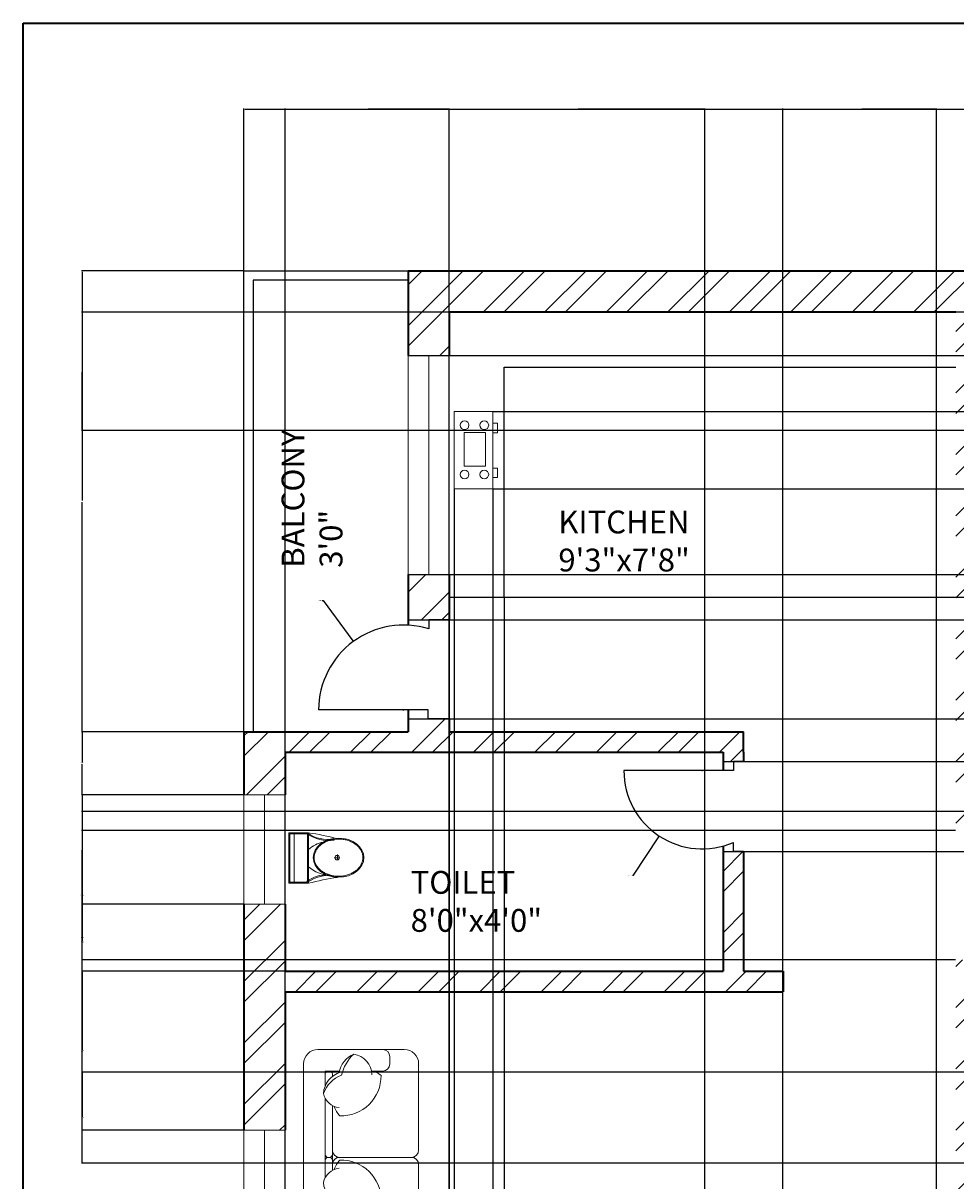
# Model space of a CAD drawing. Units: inches. Extents: x 2529 to 3014, y 1203 to 2262.
# Tile 10 of 13: x 2529 to 2733, y 2008 to 2262. Entities that reach past the tile are written whole.
import ezdxf

# ---------------------------------------------------------------- set-up
doc = ezdxf.new("R2010")
doc.units = ezdxf.units.IN
for name, color, linetype, lineweight in [('A-ANNO-DIMS', 2, 'Continuous', 18), ('A-ANNO-TTLB', 7, 'Continuous', 35), ('A-AREA-IDEN', 7, 'Continuous', 18), ('A-DOOR', 21, 'Continuous', 25), ('A-EQPM', 8, 'Continuous', 18), ('A-FLOR-CASE', 7, 'Continuous', 25), ('A-FLOR-FIXT', 8, 'Continuous', 18), ('A-FLOR-RAIL', 61, 'Continuous', 25), ('A-FURN', 8, 'Continuous', 18), ('A-GLAZ', 191, 'Continuous', 18), ('A-WALL', 7, 'Continuous', 35), ('A-WALL-PATT', 143, 'Continuous', 13)]:
    doc.layers.add(name, color=color, linetype=linetype, lineweight=lineweight)
doc.styles.get("Standard").update_dxf_attribs({"font": 'arial.ttf'})
doc.dimstyles.get("Standard").update_dxf_attribs({"dimtxt": 0.18, "dimasz": 0.18, "dimexe": 0.18, "dimexo": 0.0625, "dimgap": 0.09, "dimtad": 0, "dimtih": 1, "dimtoh": 1, "dimdec": 4, "dimzin": 0, "dimdsep": 46, "dimtxsty": 'Standard', "dimcen": 0.09, "dimadec": 0, "dimazin": 0, "dimtfac": 1, "dimtdec": 4, "dimtofl": 0, "dimtmove": 0, "dimatfit": 3, "dimfxl": 1, "dimtolj": 1, "dimtzin": 0, "dimarcsym": 0})

# ---------------------------------------------------------------- blocks, each defined once
blk = doc.blocks.new('A$C31115884')
for p, q in [((283, 498), (223, 498)), ((258, 466), (258, 523)), ((0, 200), (0, 0)), ((520, 200), (0, 200)), ((10, 190), (10, 10)), ((510, 190), (10, 190)), ((510, 10), (510, 190)), ((520, 0), (520, 200)), ((510, 54), (0, 54)), ((10, 10), (510, 10)), ((0, 0), (520, 0))]:
    blk.add_line(p, q)
blk.add_circle((256, 496), 23.6)
for centre, radius, start, end in [((2778, -205), 2807, 165.4549, 171.7133), ((3237, 905), 2807, 188.2867, 194.5451), ((-295, 403), 365, 324.2091, 9.3499), ((-295, 403), 375, 324.2091, 9.3499), ((139, 406), 293, 315.8436, 2.6563), ((806, 403), 375, 179.2036, 215.7909), ((806, 403), 365, 170.6501, 215.7909), ((384, 406), 293, 190.2774, 224.1564)]:
    blk.add_arc(centre, radius, start, end)
blk.add_ellipse((256, 510), major_axis=(0, -261), ratio=0.772727)
blk.add_open_spline([(256, 259), (263, 259), (270, 260), (288, 262), (299, 265), (320, 273), (330, 278), (350, 291), (360, 299), (378, 316), (386, 326), (402, 347), (409, 358), (421, 383), (427, 395), (436, 422), (440, 436), (445, 465), (447, 480), (448, 509), (448, 524), (445, 553), (443, 568), (436, 596), (432, 610), (422, 636), (416, 649), (402, 672), (395, 683), (379, 703), (370, 712), (351, 728), (341, 735), (321, 746), (310, 751), (289, 757), (278, 759), (256, 761), (245, 761), (223, 757), (212, 754), (191, 746), (181, 741), (161, 728), (151, 720), (133, 703), (125, 693), (110, 672), (103, 660), (90, 636), (85, 623), (76, 596), (72, 582), (67, 553), (66, 538), (64, 509), (65, 494), (68, 465), (70, 450), (77, 422), (81, 408), (91, 382), (97, 370), (111, 346), (118, 335), (135, 316), (144, 307), (162, 291), (172, 284), (193, 273), (203, 269), (225, 262), (236, 260), (250, 259), (253, 259), (256, 259)], degree=3, knots=[0, 0, 0, 0, 0.110105, 0.110105, 0.285049, 0.285049, 0.459994, 0.459994, 0.634938, 0.634938, 0.809882, 0.809882, 0.984827, 0.984827, 1.159771, 1.159771, 1.334715, 1.334715, 1.50966, 1.50966, 1.684604, 1.684604, 1.859549, 1.859549, 2.034493, 2.034493, 2.209437, 2.209437, 2.384382, 2.384382, 2.559326, 2.559326, 2.73427, 2.73427, 2.909215, 2.909215, 3.084159, 3.084159, 3.259103, 3.259103, 3.434048, 3.434048, 3.608992, 3.608992, 3.783936, 3.783936, 3.958881, 3.958881, 4.133825, 4.133825, 4.30877, 4.30877, 4.483714, 4.483714, 4.658658, 4.658658, 4.833603, 4.833603, 5.008547, 5.008547, 5.183491, 5.183491, 5.358436, 5.358436, 5.53338, 5.53338, 5.708324, 5.708324, 5.883269, 5.883269, 6.058213, 6.058213, 6.233158, 6.233158, 6.283185, 6.283185, 6.283185, 6.283185])
blk = doc.blocks.new('WIN-60x9')
for p, q in [((0, 60), (9, 60)), ((0, 60), (0, 0)), ((9, 60), (4.5, 60)), ((4.5, 60), (4.5, 0)), ((9, 60), (9, 0)), ((4.5, 0), (0, 0)), ((0, 0), (9, 0))]:
    blk.add_line(p, q)
blk = doc.blocks.new('*D16')
at = {"layer": 'A-ANNO-DIMS', "color": 0, "lineweight": -2, "transparency": 16777216}
for p, q in [((2577.06, 2207.57), (2577.06, 2243.11)), ((2577.24, 2242.93), (2774.27, 2242.93)), ((2971.88, 2242.93), (2774.84, 2242.93)), ((2972.06, 2207.57), (2972.06, 2243.11))]:
    blk.add_line(p, q, dxfattribs=at)
at = {"layer": 'A-ANNO-DIMS', "color": 0, "transparency": 16777216}
for points in [[(2577.24, 2242.96), (2577.24, 2242.9), (2577.06, 2242.93)], [(2971.88, 2242.96), (2971.88, 2242.9), (2972.06, 2242.93)]]:
    blk.add_solid(points, dxfattribs=at)
at = {"layer": 'Defpoints', "color": 0, "transparency": 16777216}
for p in [(2972.06, 2242.93), (2577.06, 2207.5), (2972.06, 2207.5)]:
    blk.add_point(p, dxfattribs=at)
at = {"layer": 'A-ANNO-DIMS', "color": 0, "transparency": 16777216, "insert": (2774.56, 2242.93), "char_height": 0.18, "attachment_point": 5}
blk.add_mtext('\\A1;395', dxfattribs=at)
blk = doc.blocks.new('*D27')
at = {"layer": 'A-ANNO-DIMS', "color": 0, "lineweight": -2, "transparency": 16777216}
for p, q in [((2585.99, 2054), (2541.45, 2054)), ((2541.63, 2053.82), (2541.63, 2036.75)), ((2541.63, 2019.3), (2541.63, 2036.38)), ((2576.99, 2019.12), (2541.45, 2019.12))]:
    blk.add_line(p, q, dxfattribs=at)
at = {"layer": 'A-ANNO-DIMS', "color": 0, "transparency": 16777216}
for points in [[(2541.6, 2053.82), (2541.66, 2053.82), (2541.63, 2054)], [(2541.6, 2019.3), (2541.66, 2019.3), (2541.63, 2019.12)]]:
    blk.add_solid(points, dxfattribs=at)
at = {"layer": 'Defpoints', "color": 0, "transparency": 16777216}
for p in [(2541.63, 2054), (2586.06, 2054), (2577.06, 2019.12)]:
    blk.add_point(p, dxfattribs=at)
at = {"layer": 'A-ANNO-DIMS', "color": 0, "transparency": 16777216, "insert": (2541.63, 2036.56), "char_height": 0.18, "attachment_point": 5}
blk.add_mtext('\\A1;34.88', dxfattribs=at)
blk = doc.blocks.new('*D28')
at = {"layer": 'A-ANNO-DIMS', "color": 0, "lineweight": -2, "transparency": 16777216}
for p, q in [((2576.99, 2068.69), (2541.45, 2068.69)), ((2541.63, 2068.51), (2541.63, 2061.53)), ((2541.63, 2054.18), (2541.63, 2061.17)), ((2585.99, 2054), (2541.45, 2054))]:
    blk.add_line(p, q, dxfattribs=at)
at = {"layer": 'A-ANNO-DIMS', "color": 0, "transparency": 16777216}
for points in [[(2541.6, 2068.51), (2541.66, 2068.51), (2541.63, 2068.69)], [(2541.6, 2054.18), (2541.66, 2054.18), (2541.63, 2054)]]:
    blk.add_solid(points, dxfattribs=at)
at = {"layer": 'Defpoints', "color": 0, "transparency": 16777216}
for p in [(2541.63, 2068.69), (2577.06, 2068.69), (2586.06, 2054)]:
    blk.add_point(p, dxfattribs=at)
at = {"layer": 'A-ANNO-DIMS', "color": 0, "transparency": 16777216, "insert": (2541.63, 2061.35), "char_height": 0.18, "attachment_point": 5}
blk.add_mtext('\\A1;14.69', dxfattribs=at)
blk = doc.blocks.new('*D29')
at = {"layer": 'A-ANNO-DIMS', "color": 0, "lineweight": -2, "transparency": 16777216}
for p, q in [((2576.99, 2092.69), (2541.45, 2092.69)), ((2541.63, 2092.51), (2541.63, 2080.87)), ((2541.63, 2068.87), (2541.63, 2080.51)), ((2576.99, 2068.69), (2541.45, 2068.69))]:
    blk.add_line(p, q, dxfattribs=at)
at = {"layer": 'A-ANNO-DIMS', "color": 0, "transparency": 16777216}
for points in [[(2541.6, 2092.51), (2541.66, 2092.51), (2541.63, 2092.69)], [(2541.6, 2068.87), (2541.66, 2068.87), (2541.63, 2068.69)]]:
    blk.add_solid(points, dxfattribs=at)
at = {"layer": 'Defpoints', "color": 0, "transparency": 16777216}
for p in [(2541.63, 2092.69), (2577.06, 2092.69), (2577.06, 2068.69)]:
    blk.add_point(p, dxfattribs=at)
at = {"layer": 'A-ANNO-DIMS', "color": 0, "transparency": 16777216, "insert": (2541.63, 2080.69), "char_height": 0.18, "attachment_point": 5}
blk.add_mtext('\\A1;24', dxfattribs=at)
blk = doc.blocks.new('*D30')
at = {"layer": 'A-ANNO-DIMS', "color": 0, "lineweight": -2, "transparency": 16777216}
for p, q in [((2576.99, 2106.5), (2541.45, 2106.5)), ((2541.63, 2106.32), (2541.63, 2099.78)), ((2541.63, 2092.87), (2541.63, 2099.42)), ((2576.99, 2092.69), (2541.45, 2092.69))]:
    blk.add_line(p, q, dxfattribs=at)
at = {"layer": 'A-ANNO-DIMS', "color": 0, "transparency": 16777216}
for points in [[(2541.6, 2106.32), (2541.66, 2106.32), (2541.63, 2106.5)], [(2541.6, 2092.87), (2541.66, 2092.87), (2541.63, 2092.69)]]:
    blk.add_solid(points, dxfattribs=at)
at = {"layer": 'Defpoints', "color": 0, "transparency": 16777216}
for p in [(2541.63, 2106.5), (2577.06, 2106.5), (2577.06, 2092.69)]:
    blk.add_point(p, dxfattribs=at)
at = {"layer": 'A-ANNO-DIMS', "color": 0, "transparency": 16777216, "insert": (2541.63, 2099.6), "char_height": 0.18, "attachment_point": 5}
blk.add_mtext('\\A1;13.811', dxfattribs=at)
blk = doc.blocks.new('*D31')
at = {"layer": 'A-ANNO-DIMS', "color": 0, "lineweight": -2, "transparency": 16777216}
for p, q in [((2576.99, 2207.5), (2541.45, 2207.5)), ((2541.63, 2207.32), (2541.63, 2157.19)), ((2541.63, 2106.68), (2541.63, 2156.82)), ((2576.99, 2106.5), (2541.45, 2106.5))]:
    blk.add_line(p, q, dxfattribs=at)
at = {"layer": 'A-ANNO-DIMS', "color": 0, "transparency": 16777216}
for points in [[(2541.6, 2207.32), (2541.66, 2207.32), (2541.63, 2207.5)], [(2541.6, 2106.68), (2541.66, 2106.68), (2541.63, 2106.5)]]:
    blk.add_solid(points, dxfattribs=at)
at = {"layer": 'Defpoints', "color": 0, "transparency": 16777216}
for p in [(2541.63, 2207.5), (2577.06, 2207.5), (2577.06, 2106.5)]:
    blk.add_point(p, dxfattribs=at)
at = {"layer": 'A-ANNO-DIMS', "color": 0, "transparency": 16777216, "insert": (2541.63, 2157), "char_height": 0.18, "attachment_point": 5}
blk.add_mtext('\\A1;101', dxfattribs=at)
blk = doc.blocks.new('*D32')
at = {"layer": 'A-ANNO-DIMS', "color": 0, "lineweight": -2, "transparency": 16777216}
for p, q in [((2586.06, 1826.63), (2586.06, 2243.11)), ((2586.24, 2242.93), (2603.84, 2242.93)), ((2621.88, 2242.93), (2604.27, 2242.93)), ((2622.06, 1826.63), (2622.06, 2243.11))]:
    blk.add_line(p, q, dxfattribs=at)
at = {"layer": 'A-ANNO-DIMS', "color": 0, "transparency": 16777216}
for points in [[(2586.24, 2242.96), (2586.24, 2242.9), (2586.06, 2242.93)], [(2621.88, 2242.96), (2621.88, 2242.9), (2622.06, 2242.93)]]:
    blk.add_solid(points, dxfattribs=at)
at = {"layer": 'Defpoints', "color": 0, "transparency": 16777216}
for p in [(2622.06, 2242.93), (2586.06, 1826.57), (2622.06, 1826.57)]:
    blk.add_point(p, dxfattribs=at)
at = {"layer": 'A-ANNO-DIMS', "color": 0, "transparency": 16777216, "insert": (2604.06, 2242.93), "char_height": 0.18, "attachment_point": 5}
blk.add_mtext('\\A1;36', dxfattribs=at)
blk = doc.blocks.new('*D46')
at = {"layer": 'A-ANNO-DIMS', "color": 0, "lineweight": -2, "transparency": 16777216}
for p, q in [((2613.12, 2188.94), (3007.66, 2188.94)), ((3007.48, 2188.76), (3007.48, 2165.12)), ((3007.48, 2141.12), (3007.48, 2164.75)), ((2613.12, 2140.94), (3007.66, 2140.94))]:
    blk.add_line(p, q, dxfattribs=at)
at = {"layer": 'A-ANNO-DIMS', "color": 0, "transparency": 16777216}
for points in [[(3007.45, 2188.76), (3007.51, 2188.76), (3007.48, 2188.94)], [(3007.45, 2141.12), (3007.51, 2141.12), (3007.48, 2140.94)]]:
    blk.add_solid(points, dxfattribs=at)
at = {"layer": 'Defpoints', "color": 0, "transparency": 16777216}
for p in [(2613.06, 2188.94), (3007.48, 2188.94), (2613.06, 2140.94)]:
    blk.add_point(p, dxfattribs=at)
at = {"layer": 'A-ANNO-DIMS', "color": 0, "transparency": 16777216, "insert": (3007.48, 2164.94), "char_height": 0.18, "attachment_point": 5}
blk.add_mtext('\\A1;48', dxfattribs=at)
blk = doc.blocks.new('*D47')
at = {"layer": 'A-ANNO-DIMS', "color": 0, "lineweight": -2, "transparency": 16777216}
for p, q in [((2622.12, 2131.02), (3007.66, 2131.02)), ((3007.48, 2130.84), (3007.48, 2120.34)), ((3007.48, 2109.48), (3007.48, 2119.98)), ((2622.12, 2109.3), (3007.66, 2109.3))]:
    blk.add_line(p, q, dxfattribs=at)
at = {"layer": 'A-ANNO-DIMS', "color": 0, "transparency": 16777216}
for points in [[(3007.45, 2130.84), (3007.51, 2130.84), (3007.48, 2131.02)], [(3007.45, 2109.48), (3007.51, 2109.48), (3007.48, 2109.3)]]:
    blk.add_solid(points, dxfattribs=at)
at = {"layer": 'Defpoints', "color": 0, "transparency": 16777216}
for p in [(2622.06, 2131.02), (3007.48, 2131.02), (2622.06, 2109.3)]:
    blk.add_point(p, dxfattribs=at)
at = {"layer": 'A-ANNO-DIMS', "color": 0, "transparency": 16777216, "insert": (3007.48, 2120.16), "char_height": 0.18, "attachment_point": 5}
blk.add_mtext('\\A1;21.72', dxfattribs=at)
blk = doc.blocks.new('*D48')
at = {"layer": 'A-ANNO-DIMS', "color": 0, "lineweight": -2, "transparency": 16777216}
for p, q in [((2686.62, 2099.98), (3007.66, 2099.98)), ((3007.48, 2099.8), (3007.48, 2090.29)), ((3007.48, 2080.41), (3007.48, 2089.93)), ((2686.62, 2080.23), (3007.66, 2080.23))]:
    blk.add_line(p, q, dxfattribs=at)
at = {"layer": 'A-ANNO-DIMS', "color": 0, "transparency": 16777216}
for points in [[(3007.45, 2099.8), (3007.51, 2099.8), (3007.48, 2099.98)], [(3007.45, 2080.41), (3007.51, 2080.41), (3007.48, 2080.23)]]:
    blk.add_solid(points, dxfattribs=at)
at = {"layer": 'Defpoints', "color": 0, "transparency": 16777216}
for p in [(2686.56, 2099.98), (3007.48, 2099.98), (2686.56, 2080.23)]:
    blk.add_point(p, dxfattribs=at)
at = {"layer": 'A-ANNO-DIMS', "color": 0, "transparency": 16777216, "insert": (3007.48, 2090.11), "char_height": 0.18, "attachment_point": 5}
blk.add_mtext('\\A1;19.75', dxfattribs=at)
blk = doc.blocks.new('*D49')
at = {"layer": 'A-ANNO-DIMS', "color": 0, "lineweight": -2, "transparency": 16777216}
for p, q in [((2732.99, 2084.81), (2541.45, 2084.81)), ((2541.63, 2084.63), (2541.63, 2070.83)), ((2541.63, 2056.67), (2541.63, 2070.47)), ((2732.99, 2056.49), (2541.45, 2056.49))]:
    blk.add_line(p, q, dxfattribs=at)
at = {"layer": 'A-ANNO-DIMS', "color": 0, "transparency": 16777216}
for points in [[(2541.6, 2084.63), (2541.66, 2084.63), (2541.63, 2084.81)], [(2541.6, 2056.67), (2541.66, 2056.67), (2541.63, 2056.49)]]:
    blk.add_solid(points, dxfattribs=at)
at = {"layer": 'Defpoints', "color": 0, "transparency": 16777216}
for p in [(2541.63, 2084.81), (2733.06, 2084.81), (2733.06, 2056.49)]:
    blk.add_point(p, dxfattribs=at)
at = {"layer": 'A-ANNO-DIMS', "color": 0, "transparency": 16777216, "insert": (2541.63, 2070.65), "char_height": 0.18, "attachment_point": 5}
blk.add_mtext('\\A1;28.316', dxfattribs=at)
blk = doc.blocks.new('*D52')
at = {"layer": 'A-ANNO-DIMS', "color": 0, "lineweight": -2, "transparency": 16777216}
for p, q in [((2695.12, 1917.57), (2695.12, 2243.11)), ((2695.3, 2242.93), (2711.5, 2242.93)), ((2728.62, 2242.93), (2712.42, 2242.93)), ((2728.8, 1917.57), (2728.8, 2243.11))]:
    blk.add_line(p, q, dxfattribs=at)
at = {"layer": 'A-ANNO-DIMS', "color": 0, "transparency": 16777216}
for points in [[(2695.3, 2242.96), (2695.3, 2242.9), (2695.12, 2242.93)], [(2728.62, 2242.96), (2728.62, 2242.9), (2728.8, 2242.93)]]:
    blk.add_solid(points, dxfattribs=at)
at = {"layer": 'Defpoints', "color": 0, "transparency": 16777216}
for p in [(2728.8, 2242.93), (2695.12, 1917.5), (2728.8, 1917.5)]:
    blk.add_point(p, dxfattribs=at)
at = {"layer": 'A-ANNO-DIMS', "color": 0, "transparency": 16777216, "insert": (2711.96, 2242.93), "char_height": 0.18, "attachment_point": 5}
blk.add_mtext('\\A1;33.673', dxfattribs=at)
blk = doc.blocks.new('*D54')
at = {"layer": 'A-ANNO-DIMS', "color": 0, "lineweight": -2, "transparency": 16777216}
for p, q in [((2866.49, 2198.5), (2541.45, 2198.5)), ((2541.63, 2198.32), (2541.63, 2185.69)), ((2541.63, 2172.68), (2541.63, 2185.32)), ((2866.49, 2172.5), (2541.45, 2172.5))]:
    blk.add_line(p, q, dxfattribs=at)
at = {"layer": 'A-ANNO-DIMS', "color": 0, "transparency": 16777216}
for points in [[(2541.6, 2198.32), (2541.66, 2198.32), (2541.63, 2198.5)], [(2541.6, 2172.68), (2541.66, 2172.68), (2541.63, 2172.5)]]:
    blk.add_solid(points, dxfattribs=at)
at = {"layer": 'Defpoints', "color": 0, "transparency": 16777216}
for p in [(2541.63, 2198.5), (2866.56, 2198.5), (2866.56, 2172.5)]:
    blk.add_point(p, dxfattribs=at)
at = {"layer": 'A-ANNO-DIMS', "color": 0, "transparency": 16777216, "insert": (2541.63, 2185.5), "char_height": 0.18, "attachment_point": 5}
blk.add_mtext('\\A1;26', dxfattribs=at)
blk = doc.blocks.new('*D58')
at = {"layer": 'A-ANNO-DIMS', "color": 0, "lineweight": -2, "transparency": 16777216}
for p, q in [((2918.49, 2089), (2541.45, 2089)), ((2541.63, 2088.82), (2541.63, 2060.62)), ((2541.63, 2032.05), (2541.63, 2060.26)), ((2918.49, 2031.87), (2541.45, 2031.87))]:
    blk.add_line(p, q, dxfattribs=at)
at = {"layer": 'A-ANNO-DIMS', "color": 0, "transparency": 16777216}
for points in [[(2541.6, 2088.82), (2541.66, 2088.82), (2541.63, 2089)], [(2541.6, 2032.05), (2541.66, 2032.05), (2541.63, 2031.87)]]:
    blk.add_solid(points, dxfattribs=at)
at = {"layer": 'Defpoints', "color": 0, "transparency": 16777216}
for p in [(2918.56, 2089), (2541.63, 2031.87), (2918.56, 2031.87)]:
    blk.add_point(p, dxfattribs=at)
at = {"layer": 'A-ANNO-DIMS', "color": 0, "transparency": 16777216, "insert": (2541.63, 2060.44), "char_height": 0.18, "attachment_point": 5}
blk.add_mtext('\\A1;57.13', dxfattribs=at)
blk = doc.blocks.new('*D59')
at = {"layer": 'A-ANNO-DIMS', "color": 0, "lineweight": -2, "transparency": 16777216}
for p, q in [((2918.49, 2031.87), (2541.45, 2031.87)), ((2541.63, 2031.69), (2541.63, 2022.09)), ((2541.63, 2012.12), (2541.63, 2021.73)), ((2918.49, 2011.94), (2541.45, 2011.94))]:
    blk.add_line(p, q, dxfattribs=at)
at = {"layer": 'A-ANNO-DIMS', "color": 0, "transparency": 16777216}
for points in [[(2541.6, 2031.69), (2541.66, 2031.69), (2541.63, 2031.87)], [(2541.6, 2012.12), (2541.66, 2012.12), (2541.63, 2011.94)]]:
    blk.add_solid(points, dxfattribs=at)
at = {"layer": 'Defpoints', "color": 0, "transparency": 16777216}
for p in [(2918.56, 2031.87), (2541.63, 2011.94), (2918.56, 2011.94)]:
    blk.add_point(p, dxfattribs=at)
at = {"layer": 'A-ANNO-DIMS', "color": 0, "transparency": 16777216, "insert": (2541.63, 2021.91), "char_height": 0.18, "attachment_point": 5}
blk.add_mtext('\\A1;19.933', dxfattribs=at)
blk = doc.blocks.new('*D66')
at = {"layer": 'A-ANNO-DIMS', "color": 0, "lineweight": -2, "transparency": 16777216}
for p, q in [((2622.06, 1874.36), (2622.06, 2243.11)), ((2622.24, 2242.93), (2649.84, 2242.93)), ((2677.88, 2242.93), (2650.27, 2242.93)), ((2678.06, 1874.36), (2678.06, 2243.11))]:
    blk.add_line(p, q, dxfattribs=at)
at = {"layer": 'A-ANNO-DIMS', "color": 0, "transparency": 16777216}
for points in [[(2622.24, 2242.96), (2622.24, 2242.9), (2622.06, 2242.93)], [(2677.88, 2242.96), (2677.88, 2242.9), (2678.06, 2242.93)]]:
    blk.add_solid(points, dxfattribs=at)
at = {"layer": 'Defpoints', "color": 0, "transparency": 16777216}
for p in [(2678.06, 2242.93), (2622.06, 1874.3), (2678.06, 1874.3)]:
    blk.add_point(p, dxfattribs=at)
at = {"layer": 'A-ANNO-DIMS', "color": 0, "transparency": 16777216, "insert": (2650.06, 2242.93), "char_height": 0.18, "attachment_point": 5}
blk.add_mtext('\\A1;56', dxfattribs=at)
blk = doc.blocks.new('*D71')
at = {"layer": 'A-ANNO-DIMS', "color": 0, "lineweight": -2, "transparency": 16777216}
for p, q in [((2623.09, 2159.68), (2623.09, 1483.77)), ((2631.58, 2159.68), (2631.58, 1483.77)), ((2623.27, 1483.95), (2626.94, 1483.95)), ((2631.4, 1483.95), (2627.73, 1483.95))]:
    blk.add_line(p, q, dxfattribs=at)
at = {"layer": 'A-ANNO-DIMS', "color": 0, "transparency": 16777216}
for points in [[(2623.27, 1483.98), (2623.27, 1483.92), (2623.09, 1483.95)], [(2631.4, 1483.98), (2631.4, 1483.92), (2631.58, 1483.95)]]:
    blk.add_solid(points, dxfattribs=at)
at = {"layer": 'Defpoints', "color": 0, "transparency": 16777216}
for p in [(2623.09, 2159.75), (2631.58, 2159.75), (2631.58, 1483.95)]:
    blk.add_point(p, dxfattribs=at)
at = {"layer": 'A-ANNO-DIMS', "color": 0, "transparency": 16777216, "insert": (2627.33, 1483.95), "char_height": 0.18, "attachment_point": 5}
blk.add_mtext('\\A1;8.484', dxfattribs=at)
blk = doc.blocks.new('*D72')
at = {"layer": 'A-ANNO-DIMS', "color": 0, "lineweight": -2, "transparency": 16777216}
for p, q in [((2631.64, 2176.7), (3007.66, 2176.7)), ((3007.48, 2176.52), (3007.48, 2168.41)), ((3007.48, 2159.93), (3007.48, 2168.04)), ((2631.64, 2159.75), (3007.66, 2159.75))]:
    blk.add_line(p, q, dxfattribs=at)
at = {"layer": 'A-ANNO-DIMS', "color": 0, "transparency": 16777216}
for points in [[(3007.45, 2176.52), (3007.51, 2176.52), (3007.48, 2176.7)], [(3007.45, 2159.93), (3007.51, 2159.93), (3007.48, 2159.75)]]:
    blk.add_solid(points, dxfattribs=at)
at = {"layer": 'Defpoints', "color": 0, "transparency": 16777216}
for p in [(2631.58, 2176.7), (3007.48, 2176.7), (2631.58, 2159.75)]:
    blk.add_point(p, dxfattribs=at)
at = {"layer": 'A-ANNO-DIMS', "color": 0, "transparency": 16777216, "insert": (3007.48, 2168.22), "char_height": 0.18, "attachment_point": 5}
blk.add_mtext('\\A1;16.957', dxfattribs=at)
blk = doc.blocks.new('*D73')
at = {"layer": 'A-ANNO-DIMS', "color": 0, "lineweight": -2, "transparency": 16777216}
for p, q in [((2631.64, 2159.75), (3007.66, 2159.75)), ((3007.48, 2159.57), (3007.48, 2148.04)), ((3007.48, 2136.16), (3007.48, 2147.68)), ((2634.12, 2135.98), (3007.66, 2135.98))]:
    blk.add_line(p, q, dxfattribs=at)
at = {"layer": 'A-ANNO-DIMS', "color": 0, "transparency": 16777216}
for points in [[(3007.45, 2159.57), (3007.51, 2159.57), (3007.48, 2159.75)], [(3007.45, 2136.16), (3007.51, 2136.16), (3007.48, 2135.98)]]:
    blk.add_solid(points, dxfattribs=at)
at = {"layer": 'Defpoints', "color": 0, "transparency": 16777216}
for p in [(2631.58, 2159.75), (2634.06, 2135.98), (3007.48, 2135.98)]:
    blk.add_point(p, dxfattribs=at)
at = {"layer": 'A-ANNO-DIMS', "color": 0, "transparency": 16777216, "insert": (3007.48, 2147.86), "char_height": 0.18, "attachment_point": 5}
blk.add_mtext('\\A1;23.77', dxfattribs=at)
blk = doc.blocks.new('*D74')
at = {"layer": 'A-ANNO-DIMS', "color": 0, "lineweight": -2, "transparency": 16777216}
for p, q in [((2622.06, 2135.91), (2622.06, 1483.77)), ((2634.06, 2135.91), (2634.06, 1483.77)), ((2622.24, 1483.95), (2627.6, 1483.95)), ((2633.88, 1483.95), (2628.51, 1483.95))]:
    blk.add_line(p, q, dxfattribs=at)
at = {"layer": 'A-ANNO-DIMS', "color": 0, "transparency": 16777216}
for points in [[(2622.24, 1483.98), (2622.24, 1483.92), (2622.06, 1483.95)], [(2633.88, 1483.98), (2633.88, 1483.92), (2634.06, 1483.95)]]:
    blk.add_solid(points, dxfattribs=at)
at = {"layer": 'Defpoints', "color": 0, "transparency": 16777216}
for p in [(2622.06, 2135.98), (2634.06, 2135.98), (2634.06, 1483.95)]:
    blk.add_point(p, dxfattribs=at)
at = {"layer": 'A-ANNO-DIMS', "color": 0, "transparency": 16777216, "insert": (2628.06, 1483.95), "char_height": 0.18, "attachment_point": 5}
blk.add_mtext('\\A1;12.002', dxfattribs=at)
blk = doc.blocks.new('*D89')
at = {"layer": 'A-ANNO-DIMS', "color": 0, "lineweight": -2, "transparency": 16777216}
for p, q in [((2594.23, 2135.25), (2594.41, 2135.25)), ((2594.41, 2135.25), (2600.9, 2126.41)), ((2611.99, 2111.21), (2611.99, 2111.39)), ((2611.9, 2111.3), (2612.08, 2111.3))]:
    blk.add_line(p, q, dxfattribs=at)
at = {"layer": 'A-ANNO-DIMS', "color": 0, "transparency": 16777216}
blk.add_solid([(2600.92, 2126.43), (2600.87, 2126.39), (2601, 2126.27)], dxfattribs=at)
at = {"layer": 'Defpoints', "color": 0, "transparency": 16777216}
for p in [(2601, 2126.27), (2611.99, 2111.3)]:
    blk.add_point(p, dxfattribs=at)
at = {"layer": 'A-ANNO-DIMS', "color": 0, "transparency": 16777216, "insert": (2593.68, 2135.25), "char_height": 0.18, "attachment_point": 5}
blk.add_mtext('\\A1;R18.572', dxfattribs=at)
blk = doc.blocks.new('*D93')
at = {"layer": 'A-ANNO-DIMS', "color": 0, "lineweight": -2, "transparency": 16777216}
for p, q in [((2677.38, 2097.98), (2677.56, 2097.98)), ((2677.47, 2097.89), (2677.47, 2098.07)), ((2662.4, 2075.02), (2667.95, 2083.48)), ((2662.22, 2075.02), (2662.4, 2075.02))]:
    blk.add_line(p, q, dxfattribs=at)
at = {"layer": 'A-ANNO-DIMS', "color": 0, "transparency": 16777216}
blk.add_solid([(2667.93, 2083.5), (2667.98, 2083.46), (2668.05, 2083.63)], dxfattribs=at)
at = {"layer": 'Defpoints', "color": 0, "transparency": 16777216}
for p in [(2677.47, 2097.98), (2668.05, 2083.63)]:
    blk.add_point(p, dxfattribs=at)
at = {"layer": 'A-ANNO-DIMS', "color": 0, "transparency": 16777216, "insert": (2661.74, 2075.02), "char_height": 0.18, "attachment_point": 5}
blk.add_mtext('\\A1;R17.17', dxfattribs=at)

msp = doc.modelspace()

# ---------------------------------------------------------------- hatches: boundary and pattern name
at = {"layer": 'A-WALL-PATT'}
h = msp.add_hatch(dxfattribs=at)
h.set_pattern_fill('ANSI32', color=256)
h.paths.add_polyline_path([(2686.5554, 2106.5032), (2622.0554, 2106.5032), (2622.0554, 2109.2964), (2617.4223, 2109.2964), (2613.0554, 2109.2964), (2613.0554, 2106.5032), (2577.0554, 2106.5032), (2577.0554, 2092.6918), (2586.0554, 2092.6918), (2586.0554, 2102.0032), (2682.0554, 2102.0032), (2682.0554, 2099.9833), (2686.5554, 2099.9833), (2686.5554, 2102.0032)])
h.paths.add_polyline_path([(2695.2249, 2054.0032), (2686.5554, 2054.0032), (2686.5554, 2080.2316), (2684.3054, 2080.2316), (2682.0554, 2080.2316), (2682.0554, 2054.0032), (2586.0554, 2054.0032), (2586.0554, 2068.6918), (2577.0554, 2068.6918), (2577.0554, 2019.1229), (2586.0554, 2019.1229), (2586.0554, 2049.5032), (2695.2249, 2049.5032)])
h.paths.add_polyline_path([(2737.5554, 2049.5032), (2866.5554, 2049.5032), (2866.5554, 2045.0233), (2871.0554, 2045.0233), (2871.0554, 2049.5032), (2871.0554, 2172.5032), (2866.5554, 2172.5032), (2829.1265, 2172.5032), (2829.1265, 2168.0032), (2866.5554, 2168.0032), (2866.5554, 2054.0032), (2737.5554, 2054.0032), (2737.5554, 2056.4892), (2735.3054, 2056.4892), (2733.0554, 2056.4892), (2733.0554, 2049.5032), (2733.0554, 1917.5032), (2733.0554, 1913.0032), (2871.0554, 1913.0032), (2871.0554, 1924.9149), (2868.8054, 1924.9149), (2866.5554, 1924.9149), (2866.5554, 1917.5032), (2737.5554, 1917.5032)], flags=17)
h.paths.add_polyline_path([(2972.0554, 2207.5032), (2613.0554, 2207.5032), (2613.0554, 2205.5032), (2613.0554, 2188.9366), (2622.0554, 2188.9366), (2622.0554, 2198.5032), (2733.0554, 2198.5032), (2733.0554, 2084.8053), (2735.3054, 2084.8053), (2737.5554, 2084.8053), (2737.5554, 2168.0032), (2769.1265, 2168.0032), (2769.1265, 2170.2532), (2769.1265, 2172.5032), (2737.5554, 2172.5032), (2737.5554, 2198.5032), (2963.0554, 2198.5032), (2963.0554, 2093.5032), (2912.0586, 2093.5032), (2912.0586, 2089.0032), (2918.5554, 2089.0032), (2918.5554, 2031.8749), (2923.0554, 2031.8749), (2923.0554, 2089.0032), (2963.0554, 2089.0032), (2963.0554, 2010.0032), (2923.0554, 2010.0032), (2923.0554, 2011.9417), (2918.5554, 2011.9417), (2918.5554, 2003.1338), (2923.0554, 2003.1338), (2923.0554, 2005.5032), (2963.0554, 2005.5032), (2963.0554, 1917.5032), (2963.0554, 1691.0776), (2972.0554, 1691.0776), (2972.0554, 1917.5032)])
h.paths.add_polyline_path([(2963.0554, 1945.5032), (2923.0554, 1945.5032), (2923.0554, 1983.0571), (2920.8054, 1983.0571), (2918.5554, 1983.0571), (2918.5554, 1941.0032), (2963.0554, 1941.0032)], flags=17)
h.paths.add_polyline_path([(2930.3679, 1788.7532), (2930.3679, 1791.0032), (2894.8637, 1791.0032), (2894.8637, 1786.5032), (2900.5554, 1786.5032), (2900.5554, 1784.6931), (2905.0554, 1784.6931), (2905.0554, 1786.5032), (2930.3679, 1786.5032)], flags=17)
h.paths.add_polyline_path([(2963.0554, 1791.0032), (2954.3679, 1791.0032), (2954.3679, 1786.5032), (2963.0554, 1786.5032)], flags=17)
h.paths.add_polyline_path([(2871.0554, 1853.0032), (2919.0554, 1853.0032), (2919.0554, 1847.0972), (2923.5554, 1847.0972), (2923.5554, 1853.0032), (2923.5554, 1857.5032), (2871.0554, 1857.5032), (2871.0554, 1871.7024), (2866.5554, 1871.7024), (2866.5554, 1791.0032), (2737.5554, 1791.0032), (2737.5554, 1806.6712), (2735.3054, 1806.6712), (2733.0554, 1806.6712), (2733.0554, 1791.0032), (2733.0554, 1786.5032), (2733.0554, 1780.6235), (2737.5554, 1780.6235), (2737.5554, 1786.5032), (2872.8745, 1786.5032), (2872.8745, 1788.7532), (2872.8745, 1791.0032), (2871.0554, 1791.0032)], flags=17)
h.paths.add_polyline_path([(2844.0554, 1734.0032), (2848.2652, 1734.0032), (2848.2652, 1738.5032), (2800.0167, 1738.5032), (2800.0167, 1734.0032), (2839.5554, 1734.0032), (2839.5554, 1582.5032), (2792.3334, 1582.5032), (2792.3334, 1573.5032), (2871.4433, 1573.5032), (2871.4433, 1578.0032), (2871.4433, 1582.5032), (2844.0554, 1582.5032)])
h.paths.add_polyline_path([(2972.0554, 1631.0776), (2963.0554, 1631.0776), (2963.0554, 1582.5032), (2931.4433, 1582.5032), (2931.4433, 1573.5032), (2972.0554, 1573.5032)])
h.paths.add_polyline_path([(2756.3334, 1582.5032), (2737.5554, 1582.5032), (2737.5554, 1734.0032), (2744.3201, 1734.0032), (2744.3201, 1738.5032), (2737.5554, 1738.5032), (2737.5554, 1746.0094), (2733.0554, 1746.0094), (2733.0554, 1738.5032), (2733.0554, 1612.5032), (2728.2475, 1612.5032), (2728.2475, 1603.5032), (2733.0554, 1603.5032), (2733.0554, 1582.5032), (2733.0554, 1573.5032), (2756.3334, 1573.5032), (2756.3334, 1578.0032)])
h.paths.add_polyline_path([(2695.7662, 1612.5032), (2658.4771, 1612.5032), (2658.4771, 1603.5032), (2695.7662, 1603.5032), (2695.7662, 1608.0032)])
h.paths.add_polyline_path([(2586.0554, 1686.9483), (2577.0554, 1686.9483), (2577.0554, 1603.5032), (2598.4771, 1603.5032), (2598.4771, 1608.0032), (2598.4771, 1612.5032), (2586.0554, 1612.5032)])
h.paths.add_polyline_path([(2683.2727, 1791.0032), (2586.0554, 1791.0032), (2586.0554, 1815.6736), (2581.5554, 1815.6736), (2577.0554, 1815.6736), (2577.0554, 1746.9483), (2586.0554, 1746.9483), (2586.0554, 1786.5032), (2683.2727, 1786.5032)])
h.paths.add_polyline_path([(2586.0554, 1959.1229), (2577.0554, 1959.1229), (2577.0554, 1875.6736), (2586.0554, 1875.6736), (2586.0554, 1913.0032), (2683.2727, 1913.0032), (2683.2727, 1917.5032), (2586.0554, 1917.5032)])
h = msp.add_hatch(dxfattribs=at)
h.set_pattern_fill('ANSI32', color=256)
h.paths.add_polyline_path([(2622.0554, 2140.9366), (2613.0554, 2140.9366), (2613.0554, 2131.0168), (2622.0554, 2131.0168)])

# ---------------------------------------------------------------- linework, layer by layer
at = {"layer": 'A-ANNO-TTLB'}
msp.add_lwpolyline([(2528.6765, 2261.8165), (3013.6003, 2261.8165), (3013.6003, 1455.1523), (2528.6765, 1455.1523)], close=True, dxfattribs=at)
at = {"layer": 'A-DOOR'}
for p, q in [((2613.0554, 2131.0168), (2622.0554, 2131.0168)), ((2622.0554, 2131.0168), (2617.5554, 2131.0168)), ((2617.5554, 2131.0168), (2617.5554, 2129.0168)), ((2617.4223, 2111.2964), (2593.4223, 2111.2964)), ((2613.0554, 2109.2964), (2620.7588, 2109.2964)), ((2617.4223, 2109.2964), (2617.4223, 2111.2964)), ((2622.0554, 2109.2964), (2617.4223, 2109.2964)), ((2620.7588, 2109.2964), (2622.0554, 2109.2964)), ((2682.0554, 2099.9833), (2686.5554, 2099.9833)), ((2686.5554, 2099.9833), (2684.3054, 2099.9833)), ((2684.3054, 2099.9833), (2684.3054, 2097.9833)), ((2684.3054, 2097.9833), (2660.3054, 2097.9833)), ((2684.3054, 2080.2316), (2684.3054, 2082.2316)), ((2682.0554, 2080.2316), (2686.5554, 2080.2316)), ((2686.5554, 2080.2316), (2684.3054, 2080.2316))]:
    msp.add_line(p, q, dxfattribs=at)
for centre, radius, start, end in [((2611.9947, 2111.2964), 18.5724, 72.578326, 180), ((2677.4745, 2097.9833), 17.1691, 180, 293.444396)]:
    msp.add_arc(centre, radius, start, end, dxfattribs=at)
at = {"layer": 'A-EQPM'}
for points in [[(2623.0916, 2176.7033), (2631.5753, 2176.7033), (2631.5753, 2159.7466), (2623.0916, 2159.7466)], [(2631.5753, 2174.1109), (2632.6544, 2174.1109), (2632.6544, 2172.0102), (2631.5753, 2172.0102)], [(2625.3088, 2172.0859), (2629.985, 2172.0859), (2629.985, 2164.6861), (2625.3088, 2164.6861)], [(2631.5753, 2164.2887), (2632.6544, 2164.2887), (2632.6544, 2162.188), (2631.5753, 2162.188)]]:
    msp.add_lwpolyline(points, close=True, dxfattribs=at)
for centre in [(2625.4035, 2173.6756), (2629.72, 2173.6756), (2625.4035, 2162.8882), (2629.72, 2162.8882)]:
    msp.add_circle(centre, 0.9652, dxfattribs=at)
at = {"layer": 'A-FLOR-CASE'}
for p, q in [((2634.0572, 2135.9767), (2634.0572, 2186.4372)), ((2634.0572, 2186.4372), (2733.0554, 2186.4372)), ((2622.0554, 2135.9767), (2634.0572, 2135.9767))]:
    msp.add_line(p, q, dxfattribs=at)
at = {"layer": 'A-FLOR-RAIL'}
for p, q in [((2577.0554, 2106.5032), (2577.0554, 2207.5032)), ((2577.0554, 2207.5032), (2613.0554, 2207.5032)), ((2613.0554, 2205.5032), (2579.0554, 2205.5032)), ((2579.0554, 2205.5032), (2579.0554, 2106.5032)), ((2613.0554, 2207.5032), (2613.0554, 2205.5032))]:
    msp.add_line(p, q, dxfattribs=at)
at = {"layer": 'A-FURN', "ltscale": 0.03}
msp.add_lwpolyline([(2615.3428, 2014.7731, -0.41421356), (2613.7668, 2013.1971, -0.41421356), (2615.3428, 2011.621), (2615.3428, 1992.7085, -0.41421356), (2612.1907, 1989.5564), (2593.2781, 1989.5564, -0.41421356), (2590.126, 1992.7085), (2590.126, 2033.6857, -0.41421356), (2593.2781, 2036.8378), (2612.1907, 2036.8378, -0.41421356), (2615.3428, 2033.6857), (2615.3428, 2014.7731, -0.41421356), (2613.7668, 2013.1971, -0.41421356), (2615.3428, 2011.621)], format="xyb", dxfattribs=at)
at = {"layer": 'A-FURN'}
for points in [[(2601.1435, 2035.8348, 0.14772988), (2598.4349, 2031.2284, 0.21334276), (2594.4623, 2027.164, 0.17866181)], [(2605.1161, 2031.3187, 0.35677236), (2601.1435, 2035.8348, 0.24954205), (2597.8697, 2031.7428, -9.61688035)], [(2607.4626, 2036.8378, -0.41421356), (2609.0386, 2035.2618), (2609.0386, 2033.6857, -0.41421356), (2607.4626, 2032.1097), (2605.0207, 2032.1097)], [(2598.219, 2031.8648, 0.30666349), (2594.4623, 2027.164, 0.30632997), (2597.8932, 2024.0931, -0.87284716)], [(2596.4302, 2030.907), (2596.4302, 2031.4792, 0.41421356), (2595.7998, 2032.1097), (2595.4846, 2032.1097, 0.41421356), (2594.8542, 2031.4792)], [(2594.8542, 2031.4792), (2594.8542, 2028.7941, 0.41421356)], [(2605.02, 2032.1131, -0.16554063), (2607.1024, 2031.1381, -0.42598917), (2598.0737, 2022.2867, -0.12152332), (2596.8293, 2024.3879, 7.11546429)], [(2594.8542, 2026.1721), (2594.8542, 2013.8275, 0.41421356), (2595.4846, 2013.1971), (2595.7998, 2013.1971, 0.41421356), (2596.4302, 2013.8275), (2596.4302, 2024.5851, 0.41421356)], [(2594.8542, 2008.7122), (2594.8542, 2012.5667, -0.41421356), (2595.4846, 2013.1971), (2595.7998, 2013.1971, -0.41421356), (2596.4302, 2012.5667), (2596.4302, 2010.2991, -0.41421356)], [(2596.4302, 2014.7731, 0.41421356), (2598.0063, 2013.1971)], [(2596.4302, 2014.7731, 0.41421356), (2598.0063, 2013.1971), (2613.7668, 2013.1971, 0.41421356)], [(2596.4302, 2011.621, -0.41421356), (2598.0063, 2013.1971)], [(2596.4302, 2011.621, -0.41421356), (2598.0063, 2013.1971), (2613.7668, 2013.1971, -0.41421356)], [(2605.02, 2002.7712, 0.16554063), (2607.1024, 2003.7462, 0.42598917), (2598.0737, 2012.5976, 0.12152332), (2596.8293, 2010.4964, -7.11546429)], [(2598.219, 2003.0195, -0.30666349), (2594.4623, 2007.7203, -0.30632997), (2597.8932, 2010.7912, 0.87284716)]]:
    msp.add_lwpolyline(points, format="xyb", dxfattribs=at)
for points in [[(2597.9515, 2032.1097), (2594.8542, 2032.1097), (2594.8542, 2028.7941)], [(2594.8542, 2026.1721), (2594.8542, 2008.7122)]]:
    msp.add_lwpolyline(points, dxfattribs=at)
msp.add_lwpolyline([(2594.8542, 2013.8275), (2594.8542, 2012.5667, -0.41421356), (2595.4846, 2013.1971), (2595.7998, 2013.1971, -0.41421356), (2596.4302, 2012.5667), (2596.4302, 2013.8275, -0.41421356), (2595.7998, 2013.1971), (2595.4846, 2013.1971, -0.41421356)], format="xyb", close=True, dxfattribs=at)
at = {"layer": 'A-GLAZ'}
for p, q in [((2613.0554, 2188.9366), (2622.0554, 2188.9366)), ((2613.0554, 2188.9366), (2613.0554, 2140.9366)), ((2622.0554, 2188.9366), (2617.5554, 2188.9366)), ((2617.5554, 2188.9366), (2617.5554, 2140.9366)), ((2622.0554, 2188.9366), (2622.0554, 2140.9366)), ((2617.5554, 2140.9366), (2613.0554, 2140.9366)), ((2613.0554, 2140.9366), (2622.0554, 2140.9366)), ((2577.0554, 2092.6918), (2586.0554, 2092.6918)), ((2577.0554, 2092.6918), (2577.0554, 2068.6918)), ((2586.0554, 2092.6918), (2581.5554, 2092.6918)), ((2581.5554, 2092.6918), (2581.5554, 2068.6918)), ((2586.0554, 2068.6918), (2586.0554, 2092.6918)), ((2581.5554, 2068.6918), (2577.0554, 2068.6918)), ((2577.0554, 2068.6918), (2586.0554, 2068.6918))]:
    msp.add_line(p, q, dxfattribs=at)
at = {"layer": 'A-WALL'}
for p, q in [((2613.0554, 2207.5032), (2972.0554, 2207.5032)), ((2613.0554, 2207.5032), (2613.0554, 2188.9366)), ((2622.0554, 2198.5032), (2622.0554, 2188.9366)), ((2622.0554, 2198.5032), (2733.0554, 2198.5032)), ((2613.0554, 2140.9366), (2613.0554, 2129.8385)), ((2622.0554, 2140.9366), (2622.0554, 2131.0168)), ((2613.0554, 2111.2964), (2613.0554, 2106.5032)), ((2622.0554, 2109.2964), (2622.0554, 2106.5032)), ((2577.0554, 2106.5032), (2577.0554, 2092.6918)), ((2577.0554, 2106.5032), (2613.0554, 2106.5032)), ((2622.0554, 2106.5032), (2686.5554, 2106.5032)), ((2686.5554, 2102.0032), (2686.5554, 2106.5032)), ((2586.0554, 2102.0032), (2682.0554, 2102.0032)), ((2586.0554, 2102.0032), (2586.0554, 2092.6918)), ((2682.0554, 2102.0032), (2682.0554, 2097.9833)), ((2686.5554, 2102.0032), (2686.5554, 2099.9833)), ((2682.0554, 2081.4366), (2682.0554, 2054.0032)), ((2686.5554, 2080.2316), (2686.5554, 2054.0032)), ((2577.0554, 2068.6918), (2577.0554, 2019.1229)), ((2586.0554, 2068.6918), (2586.0554, 2054.0032)), ((2586.0554, 2054.0032), (2682.0554, 2054.0032)), ((2686.5554, 2054.0032), (2695.2249, 2054.0032)), ((2695.2249, 2054.0032), (2695.2249, 2049.5032)), ((2586.0554, 2049.5032), (2695.2249, 2049.5032)), ((2586.0554, 2049.5032), (2586.0554, 2019.1229))]:
    msp.add_line(p, q, dxfattribs=at)

# ---------------------------------------------------------------- block references
at = {"layer": 'A-FLOR-FIXT', "xscale": 0.021283599635143, "yscale": 0.021283599635143, "zscale": 0.021283599635143, "rotation": 270}
msp.add_blockref('A$C31115884', (2586.93, 2084.3446), dxfattribs=at)
at = {"layer": 'A-GLAZ'}
msp.add_blockref('WIN-60x9', (2577.055, 1959.123), dxfattribs=at)

# ---------------------------------------------------------------- texts
at = {"layer": 'A-AREA-IDEN', "insert": (2585.307, 2142.4379), "char_height": 5, "attachment_point": 1, "rotation": 90}
msp.add_mtext_dynamic_manual_height_columns('BALCONY\\P3\'0"', width=134.77658, gutter_width=12.5, heights=[0], dxfattribs=at)
at = {"layer": 'A-AREA-IDEN', "char_height": 5, "attachment_point": 1}
for s, width, insert in [('KITCHEN\\P9\'3"x7\'8"', 160.921755, (2645.9538, 2154.9666)), ('TOILET\\P8\'0"x4\'0"', 152.904571, (2613.5822, 2075.9721))]:
    msp.add_mtext_dynamic_manual_height_columns(s, width=width, gutter_width=12.5, heights=[0], dxfattribs=dict(at, insert=insert))

# ---------------------------------------------------------------- dimensions: what is measured, and where the dimension line sits
at = {"layer": 'A-ANNO-DIMS'}
for base, p1, p2, override, picture, middle in [((2972.0554, 2242.9282), (2577.0554, 2207.5032), (2972.0554, 2207.5032), {"dimdec": 0, "dimlfac": 1, "dimrnd": 0, "dimzin": 0, "dimdsep": 46, "dimlunit": 2}, '*D16', (2774.5554, 2242.9282)), ((2622.0554, 2242.9282), (2586.0554, 1826.5675), (2622.0554, 1826.5675), {"dimdec": 0, "dimlfac": 1, "dimrnd": 0, "dimzin": 0, "dimdsep": 46, "dimlunit": 2}, '*D32', (2604.0554, 2242.9282)), ((2678.0554, 2242.9282), (2622.0554, 1874.3024), (2678.0554, 1874.3024), {"dimdec": 0, "dimlfac": 1, "dimrnd": 0, "dimzin": 0, "dimdsep": 46, "dimlunit": 2}, '*D66', (2650.0554, 2242.9282)), ((2728.79627, 2242.92823), (2695.12279, 1917.50323), (2728.79627, 1917.50323), {"dimdec": 3, "dimlfac": 1, "dimrnd": 0, "dimzin": 0, "dimdsep": 46, "dimlunit": 2}, '*D52', (2711.95953, 2242.92823)), ((2631.5753, 1483.9492), (2623.0916, 2159.7466), (2631.5753, 2159.7466), {"dimdec": 3, "dimlfac": 1, "dimrnd": 0, "dimzin": 0, "dimdsep": 46, "dimlunit": 2}, '*D71', (2627.3335, 1483.9492)), ((2634.0572, 1483.9492), (2622.0554, 2135.9767), (2634.0572, 2135.9767), {"dimdec": 3, "dimlfac": 1, "dimrnd": 0, "dimzin": 0, "dimdsep": 46, "dimlunit": 2}, '*D74', (2628.0563, 1483.9492))]:
    dim = msp.add_linear_dim(base=base, p1=p1, p2=p2, dimstyle='Standard', override=override, dxfattribs=at)
    dim.commit()
    dim.dimension.update_dxf_attribs({"geometry": picture, "text_midpoint": middle})
for base, p1, p2, override, picture, middle in [((2541.6304, 2207.5032), (2577.0554, 2106.5032), (2577.0554, 2207.5032), {"dimdec": 0, "dimlfac": 1, "dimrnd": 0, "dimzin": 0, "dimdsep": 46, "dimlunit": 2}, '*D31', (2541.6304, 2157.0032)), ((2541.6304, 2198.5032), (2866.5554, 2172.5032), (2866.5554, 2198.5032), {"dimdec": 0, "dimlfac": 1, "dimrnd": 0, "dimzin": 0, "dimdsep": 46, "dimlunit": 2}, '*D54', (2541.6304, 2185.5032)), ((3007.4804, 2188.9366), (2613.0554, 2140.9366), (2613.0554, 2188.9366), {"dimdec": 0, "dimlfac": 1, "dimrnd": 0, "dimzin": 0, "dimdsep": 46, "dimlunit": 2}, '*D46', (3007.4804, 2164.9366)), ((3007.4804, 2176.7033), (2631.5753, 2159.7466), (2631.5753, 2176.7033), {"dimdec": 3, "dimlfac": 1, "dimrnd": 0, "dimzin": 0, "dimdsep": 46, "dimlunit": 2}, '*D72', (3007.4804, 2168.225)), ((3007.4804, 2135.9767), (2631.5753, 2159.7466), (2634.0572, 2135.9767), {"dimdec": 2, "dimlfac": 1, "dimrnd": 0, "dimzin": 0, "dimdsep": 46, "dimlunit": 2}, '*D73', (3007.4804, 2147.8617)), ((3007.4804, 2131.0168), (2622.0554, 2109.2964), (2622.0554, 2131.0168), {"dimdec": 2, "dimlfac": 1, "dimrnd": 0, "dimzin": 0, "dimdsep": 46, "dimlunit": 2}, '*D47', (3007.4804, 2120.1566)), ((2541.6304, 2106.5032), (2577.0554, 2092.6918), (2577.0554, 2106.5032), {"dimdec": 3, "dimlfac": 1, "dimrnd": 0, "dimzin": 0, "dimdsep": 46, "dimlunit": 2}, '*D30', (2541.6304, 2099.5975)), ((3007.4804, 2099.9833), (2686.5554, 2080.2316), (2686.5554, 2099.9833), {"dimdec": 2, "dimlfac": 1, "dimrnd": 0, "dimzin": 0, "dimdsep": 46, "dimlunit": 2}, '*D48', (3007.4804, 2090.1074)), ((2541.6304, 2092.6918), (2577.0554, 2068.6918), (2577.0554, 2092.6918), {"dimdec": 0, "dimlfac": 1, "dimrnd": 0, "dimzin": 0, "dimdsep": 46, "dimlunit": 2}, '*D29', (2541.6304, 2080.6918)), ((2541.6304, 2031.8749), (2918.5554, 2089.0032), (2918.5554, 2031.8749), {"dimdec": 2, "dimlfac": 1, "dimrnd": 0, "dimzin": 0, "dimdsep": 46, "dimlunit": 2}, '*D58', (2541.6304, 2060.4391)), ((2541.6304, 2084.8053), (2733.0554, 2056.4892), (2733.0554, 2084.8053), {"dimdec": 3, "dimlfac": 1, "dimrnd": 0, "dimzin": 0, "dimdsep": 46, "dimlunit": 2}, '*D49', (2541.6304, 2070.6472)), ((2541.6304, 2068.6918), (2586.0554, 2054.0032), (2577.0554, 2068.6918), {"dimdec": 2, "dimlfac": 1, "dimrnd": 0, "dimzin": 0, "dimdsep": 46, "dimlunit": 2}, '*D28', (2541.6304, 2061.3475)), ((2541.6304, 2054.0032), (2577.0554, 2019.1229), (2586.0554, 2054.0032), {"dimdec": 2, "dimlfac": 1, "dimrnd": 0, "dimzin": 0, "dimdsep": 46, "dimlunit": 2}, '*D27', (2541.6304, 2036.5631)), ((2541.6304, 2011.9417), (2918.5554, 2031.8749), (2918.5554, 2011.9417), {"dimdec": 3, "dimlfac": 1, "dimrnd": 0, "dimzin": 0, "dimdsep": 46, "dimlunit": 2}, '*D59', (2541.6304, 2021.9083))]:
    dim = msp.add_linear_dim(base=base, p1=p1, p2=p2, angle=90, dimstyle='Standard', override=override, dxfattribs=at)
    dim.commit()
    dim.dimension.update_dxf_attribs({"geometry": picture, "text_midpoint": middle})
for center, mpoint, override, picture, middle in [((2611.9947, 2111.2964), (2601.0024, 2126.2665), {"dimdec": 3, "dimlfac": 1, "dimrnd": 0, "dimzin": 0, "dimdsep": 46, "dimlunit": 2}, '*D89', (2593.6781, 2135.2485)), ((2677.4745, 2097.9833), (2668.0538, 2083.6296), {"dimdec": 2, "dimlfac": 1, "dimrnd": 0, "dimzin": 0, "dimdsep": 46, "dimlunit": 2}, '*D93', (2661.7415, 2075.0174))]:
    dim = msp.add_radius_dim(center=center, mpoint=mpoint, dimstyle='Standard', override=override, dxfattribs=at)
    dim.commit()
    dim.dimension.update_dxf_attribs({"geometry": picture, "text_midpoint": middle, "dimtype": 164})

doc.saveas('drawing.dxf')
